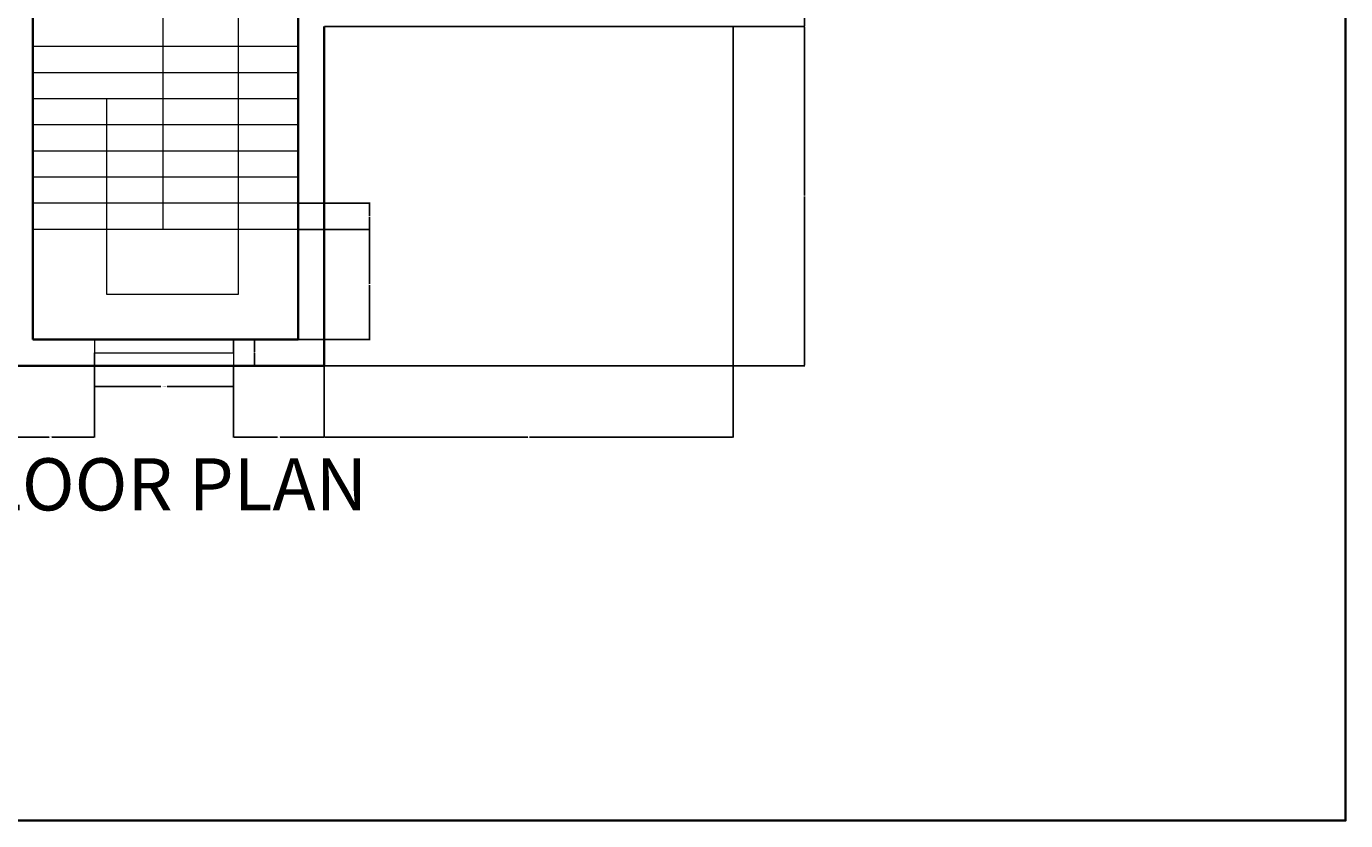
# Model space of a CAD drawing. Units: inches. Extents: x 2067 to 3463, y 1605 to 2723.
# Tile 9 of 10: x 3008 to 3463, y 1605 to 1879. Entities that reach past the tile are written whole.
import ezdxf

# ---------------------------------------------------------------- set-up
doc = ezdxf.new("R2010")
doc.units = ezdxf.units.IN
for name, color, linetype, lineweight in [('A-ANNO-DIMS', 2, 'Continuous', 18), ('A-ANNO-TEXT', 7, 'Continuous', 35), ('A-ANNO-TTLB', 7, 'Continuous', 35), ('A-FLOR-STRS', 7, 'Continuous', 18), ('A-GLAZ', 4, 'Continuous', 18), ('A-WALL', 7, 'Continuous', 35)]:
    doc.layers.add(name, color=color, linetype=linetype, lineweight=lineweight)
doc.styles.get("Standard").update_dxf_attribs({"font": 'arial.ttf'})
doc.dimstyles.get("Standard").update_dxf_attribs({"dimtxt": 0.18, "dimasz": 0.18, "dimexe": 0.18, "dimexo": 0.0625, "dimgap": 0.09, "dimtad": 0, "dimtih": 1, "dimtoh": 1, "dimdec": 4, "dimzin": 0, "dimdsep": 46, "dimtxsty": 'Standard', "dimcen": 0.09, "dimadec": 0, "dimazin": 0, "dimtfac": 1, "dimtdec": 4, "dimtofl": 0, "dimtmove": 0, "dimatfit": 3, "dimfxl": 1, "dimtolj": 1, "dimtzin": 0, "dimarcsym": 0})

# ---------------------------------------------------------------- blocks, each defined once
blk = doc.blocks.new('WIN-PLAN-48-OFFSET')
for p, q in [((0, 9), (0, 0)), ((48, 4.5), (48, 9)), ((48, 9), (48, 0)), ((0, 0), (0, 4.5)), ((0, 4.5), (48, 4.5))]:
    blk.add_line(p, q)
blk = doc.blocks.new('*D16')
at = {"layer": 'A-ANNO-DIMS', "color": 0, "lineweight": -2, "transparency": 16777216}
for p, q in [((3031.71, 1762.17), (3031.71, 1754.85)), ((3079.71, 1762.17), (3079.71, 1754.85)), ((3031.89, 1755.03), (3054.6, 1755.03)), ((3079.53, 1755.03), (3056.83, 1755.03))]:
    blk.add_line(p, q, dxfattribs=at)
at = {"layer": 'A-ANNO-DIMS', "color": 0, "transparency": 16777216}
for points in [[(3031.89, 1755.06), (3031.89, 1755), (3031.71, 1755.03)], [(3079.53, 1755.06), (3079.53, 1755), (3079.71, 1755.03)]]:
    blk.add_solid(points, dxfattribs=at)
at = {"layer": 'Defpoints', "color": 0, "transparency": 16777216}
for p in [(3031.71, 1762.23), (3079.71, 1762.23), (3079.71, 1755.03)]:
    blk.add_point(p, dxfattribs=at)
at = {"layer": 'A-ANNO-DIMS', "color": 0, "transparency": 16777216, "insert": (3055.71, 1755.03), "char_height": 0.18, "attachment_point": 5}
blk.add_mtext('\\A1;WINDOW 48 TYP.', dxfattribs=at)
blk = doc.blocks.new('*D17')
at = {"layer": 'A-ANNO-DIMS', "color": 0, "lineweight": -2, "transparency": 16777216}
for p, q in [((3079.78, 1771.23), (3087.09, 1771.23)), ((3086.91, 1771.05), (3086.91, 1766.91)), ((3086.91, 1762.41), (3086.91, 1766.55)), ((3079.78, 1762.23), (3087.09, 1762.23))]:
    blk.add_line(p, q, dxfattribs=at)
at = {"layer": 'A-ANNO-DIMS', "color": 0, "transparency": 16777216}
for points in [[(3086.88, 1771.05), (3086.94, 1771.05), (3086.91, 1771.23)], [(3086.88, 1762.41), (3086.94, 1762.41), (3086.91, 1762.23)]]:
    blk.add_solid(points, dxfattribs=at)
at = {"layer": 'Defpoints', "color": 0, "transparency": 16777216}
for p in [(3079.71, 1771.23), (3086.91, 1771.23), (3079.71, 1762.23)]:
    blk.add_point(p, dxfattribs=at)
at = {"layer": 'A-ANNO-DIMS', "color": 0, "transparency": 16777216, "insert": (3086.91, 1766.73), "char_height": 0.18, "attachment_point": 5}
blk.add_mtext('\\A1;9 TYP.', dxfattribs=at)
blk = doc.blocks.new('*D53')
at = {"layer": 'A-ANNO-DIMS', "color": 0, "lineweight": -2, "transparency": 16777216}
for p, q in [((3001.5, 1762.17), (3001.5, 1737.45)), ((3031.71, 1762.17), (3031.71, 1737.45)), ((3001.68, 1737.63), (3016.14, 1737.63)), ((3031.53, 1737.63), (3017.07, 1737.63))]:
    blk.add_line(p, q, dxfattribs=at)
at = {"layer": 'A-ANNO-DIMS', "color": 0, "transparency": 16777216}
for points in [[(3001.68, 1737.66), (3001.68, 1737.6), (3001.5, 1737.63)], [(3031.53, 1737.66), (3031.53, 1737.6), (3031.71, 1737.63)]]:
    blk.add_solid(points, dxfattribs=at)
at = {"layer": 'Defpoints', "color": 0, "transparency": 16777216}
for p in [(3001.5, 1762.23), (3031.71, 1762.23), (3031.71, 1737.63)]:
    blk.add_point(p, dxfattribs=at)
at = {"layer": 'A-ANNO-DIMS', "color": 0, "transparency": 16777216, "insert": (3016.61, 1737.63), "char_height": 0.18, "attachment_point": 5}
blk.add_mtext('\\A1;30.215', dxfattribs=at)
blk = doc.blocks.new('*D54')
at = {"layer": 'A-ANNO-DIMS', "color": 0, "lineweight": -2, "transparency": 16777216}
for p, q in [((3079.71, 1762.17), (3079.71, 1737.45)), ((3111, 1762.17), (3111, 1737.45)), ((3079.89, 1737.63), (3094.89, 1737.63)), ((3110.82, 1737.63), (3095.82, 1737.63))]:
    blk.add_line(p, q, dxfattribs=at)
at = {"layer": 'A-ANNO-DIMS', "color": 0, "transparency": 16777216}
for points in [[(3079.89, 1737.66), (3079.89, 1737.6), (3079.71, 1737.63)], [(3110.82, 1737.66), (3110.82, 1737.6), (3111, 1737.63)]]:
    blk.add_solid(points, dxfattribs=at)
at = {"layer": 'Defpoints', "color": 0, "transparency": 16777216}
for p in [(3079.71, 1762.23), (3111, 1762.23), (3111, 1737.63)]:
    blk.add_point(p, dxfattribs=at)
at = {"layer": 'A-ANNO-DIMS', "color": 0, "transparency": 16777216, "insert": (3095.36, 1737.63), "char_height": 0.18, "attachment_point": 5}
blk.add_mtext('\\A1;31.285', dxfattribs=at)
blk = doc.blocks.new('*D55')
at = {"layer": 'A-ANNO-DIMS', "color": 0, "lineweight": -2, "transparency": 16777216}
for p, q in [((3111, 1879.17), (3111, 1737.45)), ((3252, 1879.17), (3252, 1737.45)), ((3111.18, 1737.63), (3181.24, 1737.63)), ((3251.82, 1737.63), (3181.76, 1737.63))]:
    blk.add_line(p, q, dxfattribs=at)
at = {"layer": 'A-ANNO-DIMS', "color": 0, "transparency": 16777216}
for points in [[(3111.18, 1737.66), (3111.18, 1737.6), (3111, 1737.63)], [(3251.82, 1737.66), (3251.82, 1737.6), (3252, 1737.63)]]:
    blk.add_solid(points, dxfattribs=at)
at = {"layer": 'Defpoints', "color": 0, "transparency": 16777216}
for p in [(3111, 1879.23), (3252, 1879.23), (3252, 1737.63)]:
    blk.add_point(p, dxfattribs=at)
at = {"layer": 'A-ANNO-DIMS', "color": 0, "transparency": 16777216, "insert": (3181.5, 1737.63), "char_height": 0.18, "attachment_point": 5}
blk.add_mtext('\\A1;141', dxfattribs=at)
blk = doc.blocks.new('*D57')
at = {"layer": 'A-ANNO-DIMS', "color": 0, "lineweight": -2, "transparency": 16777216}
for p, q in [((3111.06, 1879.23), (3276.78, 1879.23)), ((3276.6, 1879.05), (3276.6, 1820.91)), ((3276.6, 1762.41), (3276.6, 1820.55)), ((3111.06, 1762.23), (3276.78, 1762.23))]:
    blk.add_line(p, q, dxfattribs=at)
at = {"layer": 'A-ANNO-DIMS', "color": 0, "transparency": 16777216}
for points in [[(3276.57, 1879.05), (3276.63, 1879.05), (3276.6, 1879.23)], [(3276.57, 1762.41), (3276.63, 1762.41), (3276.6, 1762.23)]]:
    blk.add_solid(points, dxfattribs=at)
at = {"layer": 'Defpoints', "color": 0, "transparency": 16777216}
for p in [(3111, 1879.23), (3276.6, 1879.23), (3111, 1762.23)]:
    blk.add_point(p, dxfattribs=at)
at = {"layer": 'A-ANNO-DIMS', "color": 0, "transparency": 16777216, "insert": (3276.6, 1820.73), "char_height": 0.18, "attachment_point": 5}
blk.add_mtext('\\A1;117', dxfattribs=at)
blk = doc.blocks.new('*D60')
at = {"layer": 'A-ANNO-DIMS', "color": 0, "lineweight": -2, "transparency": 16777216}
for p, q in [((3243.06, 1936.23), (3276.78, 1936.23)), ((3276.6, 1936.05), (3276.6, 1907.91)), ((3276.6, 1879.41), (3276.6, 1907.55)), ((3252.06, 1879.23), (3276.78, 1879.23))]:
    blk.add_line(p, q, dxfattribs=at)
at = {"layer": 'A-ANNO-DIMS', "color": 0, "transparency": 16777216}
for points in [[(3276.57, 1936.05), (3276.63, 1936.05), (3276.6, 1936.23)], [(3276.57, 1879.41), (3276.63, 1879.41), (3276.6, 1879.23)]]:
    blk.add_solid(points, dxfattribs=at)
at = {"layer": 'Defpoints', "color": 0, "transparency": 16777216}
for p in [(3243, 1936.23), (3276.6, 1936.23), (3252, 1879.23)]:
    blk.add_point(p, dxfattribs=at)
at = {"layer": 'A-ANNO-DIMS', "color": 0, "transparency": 16777216, "insert": (3276.6, 1907.73), "char_height": 0.18, "attachment_point": 5}
blk.add_mtext('\\A1;57', dxfattribs=at)
blk = doc.blocks.new('*D67')
at = {"layer": 'A-ANNO-DIMS', "color": 0, "lineweight": -2, "transparency": 16777216}
for p, q in [((3102.06, 1818.25), (3126.78, 1818.25)), ((3126.6, 1818.07), (3126.6, 1813.93)), ((3126.6, 1809.43), (3126.6, 1813.57)), ((3102.06, 1809.25), (3126.78, 1809.25))]:
    blk.add_line(p, q, dxfattribs=at)
at = {"layer": 'A-ANNO-DIMS', "color": 0, "transparency": 16777216}
for points in [[(3126.57, 1818.07), (3126.63, 1818.07), (3126.6, 1818.25)], [(3126.57, 1809.43), (3126.63, 1809.43), (3126.6, 1809.25)]]:
    blk.add_solid(points, dxfattribs=at)
at = {"layer": 'Defpoints', "color": 0, "transparency": 16777216}
for p in [(3102, 1818.25), (3102, 1809.25), (3126.6, 1809.25)]:
    blk.add_point(p, dxfattribs=at)
at = {"layer": 'A-ANNO-DIMS', "color": 0, "transparency": 16777216, "insert": (3126.6, 1813.75), "char_height": 0.18, "attachment_point": 5}
blk.add_mtext('\\A1;9', dxfattribs=at)
blk = doc.blocks.new('*D68')
at = {"layer": 'A-ANNO-DIMS', "color": 0, "lineweight": -2, "transparency": 16777216}
for p, q in [((3102.06, 1809.25), (3126.78, 1809.25)), ((3126.6, 1809.07), (3126.6, 1790.42)), ((3126.6, 1771.41), (3126.6, 1790.06)), ((3102.06, 1771.23), (3126.78, 1771.23))]:
    blk.add_line(p, q, dxfattribs=at)
at = {"layer": 'A-ANNO-DIMS', "color": 0, "transparency": 16777216}
for points in [[(3126.57, 1809.07), (3126.63, 1809.07), (3126.6, 1809.25)], [(3126.57, 1771.41), (3126.63, 1771.41), (3126.6, 1771.23)]]:
    blk.add_solid(points, dxfattribs=at)
at = {"layer": 'Defpoints', "color": 0, "transparency": 16777216}
for p in [(3102, 1809.25), (3102, 1771.23), (3126.6, 1771.23)]:
    blk.add_point(p, dxfattribs=at)
at = {"layer": 'A-ANNO-DIMS', "color": 0, "transparency": 16777216, "insert": (3126.6, 1790.24), "char_height": 0.18, "attachment_point": 5}
blk.add_mtext('\\A1;38.02', dxfattribs=at)

msp = doc.modelspace()

# ---------------------------------------------------------------- linework, layer by layer
at = {"layer": 'A-ANNO-TTLB'}
msp.add_lwpolyline([(2067.2624, 2722.6321), (3463.3053, 2722.6321), (3463.3053, 1605.3918), (2067.2624, 1605.3918)], close=True, dxfattribs=at)
at = {"layer": 'A-FLOR-STRS'}
for p, q in [((3055.4865, 1809.2531), (3055.4865, 1953.2531)), ((3081.2715, 1944.2531), (3081.2715, 1786.8304)), ((3101.9994, 1872.2531), (3010.4994, 1872.2531)), ((3101.9994, 1863.2531), (3010.4994, 1863.2531)), ((3101.9994, 1854.2531), (3010.4994, 1854.2531)), ((3035.975, 1786.8304), (3035.975, 1854.2531)), ((3101.9994, 1845.2531), (3010.4994, 1845.2531)), ((3101.9994, 1836.2531), (3010.4994, 1836.2531)), ((3101.9994, 1827.2531), (3010.4994, 1827.2531)), ((3101.9994, 1818.2531), (3010.4994, 1818.2531)), ((3101.9994, 1809.2531), (3010.4994, 1809.2531)), ((3081.2715, 1786.8304), (3035.975, 1786.8304))]:
    msp.add_line(p, q, dxfattribs=at)
at = {"layer": 'A-WALL'}
for p, q in [((3010.4994, 1957.7531), (3010.4994, 1771.2309)), ((3101.9994, 1888.2309), (3101.9994, 1771.2309)), ((3110.9994, 1879.2309), (3110.9994, 1771.2309)), ((3038.9994, 1771.2309), (3010.4994, 1771.2309)), ((3101.9994, 1771.2309), (3038.9994, 1771.2309)), ((3110.9994, 1771.2309), (3110.9994, 1762.2309)), ((3038.9994, 1762.2309), (3001.4994, 1762.2309)), ((3110.9994, 1762.2309), (3038.9994, 1762.2309))]:
    msp.add_line(p, q, dxfattribs=at)

# ---------------------------------------------------------------- block references
at = {"layer": 'A-GLAZ'}
msp.add_blockref('WIN-PLAN-48-OFFSET', (3031.714, 1762.231), dxfattribs=at)

# ---------------------------------------------------------------- texts
at = {"layer": 'A-ANNO-TEXT', "insert": (2908.6072, 1730.3295), "char_height": 18, "attachment_point": 1}
msp.add_mtext_dynamic_manual_height_columns('FIRST FLOOR PLAN', width=399.538466, gutter_width=12.5, heights=[0], dxfattribs=at)

# ---------------------------------------------------------------- dimensions: what is measured, and where the dimension line sits
at = {"layer": 'A-ANNO-DIMS'}
for base, p1, p2, angle, override, picture, middle in [((3276.5994, 1936.2309), (3251.9994, 1879.2309), (3242.9994, 1936.2309), 90, {"dimdec": 0, "dimlfac": 1, "dimrnd": 0, "dimzin": 0, "dimdsep": 46, "dimlunit": 2}, '*D60', (3276.5994, 1907.7309)), ((3276.5994, 1879.2309), (3110.9994, 1762.2309), (3110.9994, 1879.2309), 90, {"dimdec": 0, "dimlfac": 1, "dimrnd": 0, "dimzin": 0, "dimdsep": 46, "dimlunit": 2}, '*D57', (3276.5994, 1820.7309)), ((3126.5994, 1809.2531), (3101.9994, 1818.2531), (3101.9994, 1809.2531), 270, {"dimdec": 0, "dimlfac": 1, "dimrnd": 0, "dimzin": 0, "dimdsep": 46, "dimlunit": 2}, '*D67', (3126.5994, 1813.7531)), ((3126.5994, 1771.2309), (3101.9994, 1809.2531), (3101.9994, 1771.2309), 270, {"dimdec": 2, "dimlfac": 1, "dimrnd": 0, "dimzin": 0, "dimdsep": 46, "dimlunit": 2}, '*D68', (3126.5994, 1790.242))]:
    dim = msp.add_linear_dim(base=base, p1=p1, p2=p2, angle=angle, dimstyle='Standard', override=override, dxfattribs=at)
    dim.commit()
    dim.dimension.update_dxf_attribs({"geometry": picture, "text_midpoint": middle})
for base, p1, p2, override, picture, middle in [((3251.9994, 1737.6309), (3110.9994, 1879.2309), (3251.9994, 1879.2309), {"dimdec": 0, "dimlfac": 1, "dimrnd": 0, "dimzin": 0, "dimdsep": 46, "dimlunit": 2}, '*D55', (3181.4994, 1737.6309)), ((3031.7142, 1737.6309), (3001.4994, 1762.2309), (3031.7142, 1762.2309), {"dimdec": 3, "dimlfac": 1, "dimrnd": 0, "dimzin": 0, "dimdsep": 46, "dimlunit": 2}, '*D53', (3016.6068, 1737.6309)), ((3110.9994, 1737.6309), (3079.7142, 1762.2309), (3110.9994, 1762.2309), {"dimdec": 3, "dimlfac": 1, "dimrnd": 0, "dimzin": 0, "dimdsep": 46, "dimlunit": 2}, '*D54', (3095.3568, 1737.6309))]:
    dim = msp.add_linear_dim(base=base, p1=p1, p2=p2, dimstyle='Standard', override=override, dxfattribs=at)
    dim.commit()
    dim.dimension.update_dxf_attribs({"geometry": picture, "text_midpoint": middle})
dim = msp.add_linear_dim(base=(3086.9142, 1771.2309), p1=(3079.7142, 1762.2309), p2=(3079.7142, 1771.2309), angle=90, text='<> TYP.', dimstyle='Standard', override={"dimdec": 0, "dimlfac": 1, "dimrnd": 0, "dimzin": 0, "dimdsep": 46, "dimlunit": 2}, dxfattribs=at)
dim.commit()
dim.dimension.update_dxf_attribs({"geometry": '*D17', "text_midpoint": (3086.9142, 1766.7309)})
dim = msp.add_linear_dim(base=(3079.7142, 1755.0309), p1=(3031.7142, 1762.2309), p2=(3079.7142, 1762.2309), text='WINDOW <> TYP.', dimstyle='Standard', override={"dimdec": 0, "dimlfac": 1, "dimrnd": 0, "dimzin": 0, "dimdsep": 46, "dimlunit": 2}, dxfattribs=at)
dim.commit()
dim.dimension.update_dxf_attribs({"geometry": '*D16', "text_midpoint": (3055.7142, 1755.0309)})

doc.saveas('drawing.dxf')
